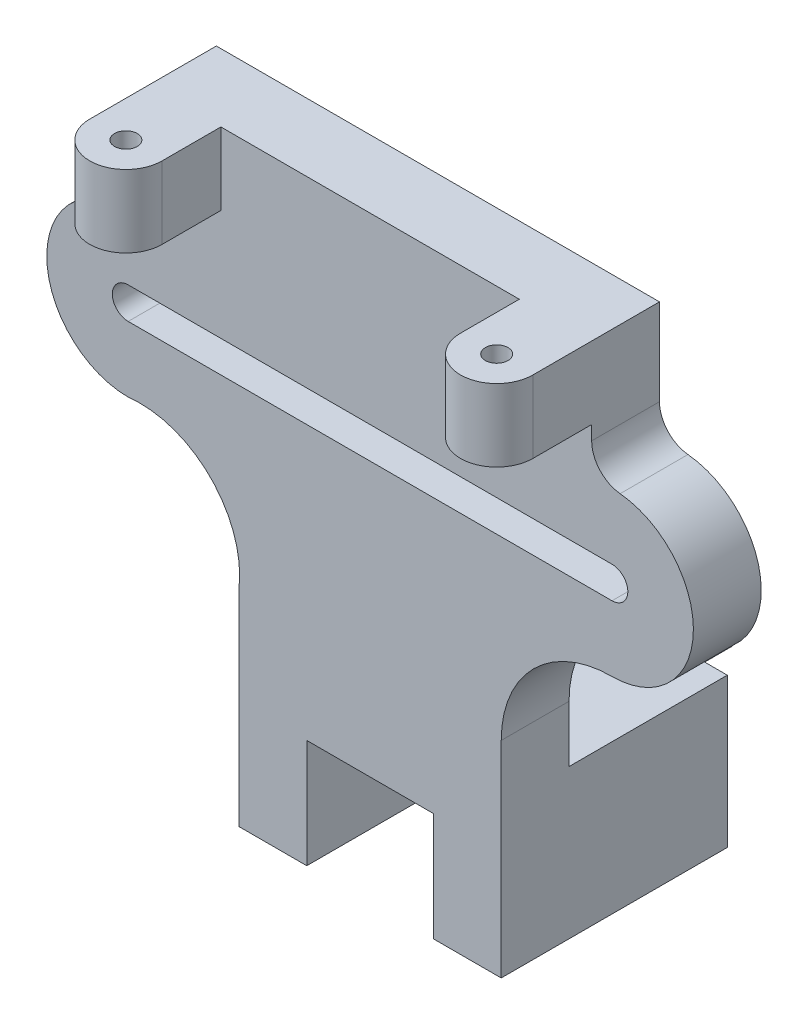
ISO-10303-21;
HEADER;
FILE_DESCRIPTION(('STEP AP214'),'2;1');
FILE_NAME('part.step','',(''),(''),'','','');
FILE_SCHEMA(('AUTOMOTIVE_DESIGN { 1 0 10303 214 1 1 1 1 }'));
ENDSEC;
DATA;
#1=APPLICATION_CONTEXT('core data for automotive mechanical design processes');
#2=APPLICATION_PROTOCOL_DEFINITION('international standard','automotive_design',2000,#1);
#3=PRODUCT_CONTEXT('',#1,'mechanical');
#4=PRODUCT('Part','Part','',(#3));
#5=PRODUCT_RELATED_PRODUCT_CATEGORY('part','',(#4));
#6=PRODUCT_DEFINITION_FORMATION('','',#4);
#7=PRODUCT_DEFINITION_CONTEXT('part definition',#1,'design');
#8=PRODUCT_DEFINITION('design','',#6,#7);
#9=PRODUCT_DEFINITION_SHAPE('','',#8);
#10=(LENGTH_UNIT() NAMED_UNIT(*) SI_UNIT(.MILLI.,.METRE.));
#11=(NAMED_UNIT(*) PLANE_ANGLE_UNIT() SI_UNIT($,.RADIAN.));
#12=(NAMED_UNIT(*) SI_UNIT($,.STERADIAN.) SOLID_ANGLE_UNIT());
#13=UNCERTAINTY_MEASURE_WITH_UNIT(LENGTH_MEASURE(1.E-05),#10,'distance_accuracy_value','');
#14=(GEOMETRIC_REPRESENTATION_CONTEXT(3) GLOBAL_UNCERTAINTY_ASSIGNED_CONTEXT((#13)) GLOBAL_UNIT_ASSIGNED_CONTEXT((#10,
#11,#12)) REPRESENTATION_CONTEXT('',''));
#15=CARTESIAN_POINT('',(0.,0.,0.));
#16=DIRECTION('',(0.,0.,1.));
#17=DIRECTION('',(1.,0.,0.));
#18=AXIS2_PLACEMENT_3D('',#15,#16,#17);
#19=CARTESIAN_POINT('',(0.,0.,0.));
#20=DIRECTION('',(0.,0.,1.));
#21=DIRECTION('',(1.,0.,0.));
#22=AXIS2_PLACEMENT_3D('',#19,#20,#21);
#23=PLANE('',#22);
#24=CARTESIAN_POINT('',(-4.5,-44.,0.));
#25=DIRECTION('',(0.,0.,1.));
#26=DIRECTION('',(1.,0.,0.));
#27=AXIS2_PLACEMENT_3D('',#24,#25,#26);
#28=CIRCLE('',#27,3.5);
#29=CARTESIAN_POINT('',(-4.5,-40.5,0.));
#30=VERTEX_POINT('',#29);
#31=CARTESIAN_POINT('',(-4.5,-47.5,0.));
#32=VERTEX_POINT('',#31);
#33=EDGE_CURVE('E390',#30,#32,#28,.T.);
#34=ORIENTED_EDGE('',*,*,#33,.T.);
#35=DIRECTION('',(1.,0.,0.));
#36=VECTOR('',#35,1.);
#37=CARTESIAN_POINT('',(0.,-47.5,0.));
#38=LINE('',#37,#36);
#39=CARTESIAN_POINT('',(102.5,-47.5,0.));
#40=VERTEX_POINT('',#39);
#41=EDGE_CURVE('E380',#32,#40,#38,.T.);
#42=ORIENTED_EDGE('',*,*,#41,.T.);
#43=CARTESIAN_POINT('',(102.5,-44.,0.));
#44=DIRECTION('',(0.,0.,1.));
#45=DIRECTION('',(1.,0.,0.));
#46=AXIS2_PLACEMENT_3D('',#43,#44,#45);
#47=CIRCLE('',#46,3.50000000000001);
#48=CARTESIAN_POINT('',(102.5,-40.5,0.));
#49=VERTEX_POINT('',#48);
#50=EDGE_CURVE('E379',#40,#49,#47,.T.);
#51=ORIENTED_EDGE('',*,*,#50,.T.);
#52=DIRECTION('',(1.,0.,0.));
#53=VECTOR('',#52,1.);
#54=CARTESIAN_POINT('',(0.,-40.5,0.));
#55=LINE('',#54,#53);
#56=EDGE_CURVE('E383',#30,#49,#55,.T.);
#57=ORIENTED_EDGE('',*,*,#56,.F.);
#58=EDGE_LOOP('',(#34,#42,#51,#57));
#59=FACE_BOUND('',#58,.T.);
#60=DIRECTION('',(0.,1.,0.));
#61=VECTOR('',#60,1.);
#62=CARTESIAN_POINT('',(78.0000000000001,0.,0.));
#63=LINE('',#62,#61);
#64=CARTESIAN_POINT('',(78.,-99.,0.));
#65=VERTEX_POINT('',#64);
#66=CARTESIAN_POINT('',(78.,-86.5,0.));
#67=VERTEX_POINT('',#66);
#68=EDGE_CURVE('E455',#65,#67,#63,.T.);
#69=ORIENTED_EDGE('',*,*,#68,.F.);
#70=DIRECTION('',(-1.,0.,0.));
#71=VECTOR('',#70,1.);
#72=CARTESIAN_POINT('',(0.,-99.,0.));
#73=LINE('',#72,#71);
#74=CARTESIAN_POINT('',(20.,-99.,0.));
#75=VERTEX_POINT('',#74);
#76=EDGE_CURVE('E47',#65,#75,#73,.T.);
#77=ORIENTED_EDGE('',*,*,#76,.T.);
#78=DIRECTION('',(0.,1.,0.));
#79=VECTOR('',#78,1.);
#80=CARTESIAN_POINT('',(20.,0.,0.));
#81=LINE('',#80,#79);
#82=CARTESIAN_POINT('',(20.,-86.5,0.));
#83=VERTEX_POINT('',#82);
#84=EDGE_CURVE('E454',#75,#83,#81,.T.);
#85=ORIENTED_EDGE('',*,*,#84,.T.);
#86=CARTESIAN_POINT('',(-1.83930843846879,-83.8458321587689,0.));
#87=DIRECTION('',(0.,0.,1.));
#88=DIRECTION('',(1.,0.,0.));
#89=AXIS2_PLACEMENT_3D('',#86,#87,#88);
#90=CIRCLE('',#89,22.);
#91=CARTESIAN_POINT('',(-2.16790270932848,-61.8482862546196,0.));
#92=VERTEX_POINT('',#91);
#93=EDGE_CURVE('E450',#92,#83,#90,.F.);
#94=ORIENTED_EDGE('',*,*,#93,.F.);
#95=CARTESIAN_POINT('',(-1.9077841989313,-83.8467484363392,0.));
#96=DIRECTION('',(0.,0.,1.));
#97=DIRECTION('',(1.,0.,0.));
#98=AXIS2_PLACEMENT_3D('',#95,#96,#97);
#99=CIRCLE('',#98,22.);
#100=CARTESIAN_POINT('',(-4.49999999999998,-62.,0.));
#101=VERTEX_POINT('',#100);
#102=EDGE_CURVE('E405',#101,#92,#99,.F.);
#103=ORIENTED_EDGE('',*,*,#102,.F.);
#104=CARTESIAN_POINT('',(-4.5,-44.,0.));
#105=DIRECTION('',(0.,0.,1.));
#106=DIRECTION('',(1.,0.,0.));
#107=AXIS2_PLACEMENT_3D('',#104,#105,#106);
#108=CIRCLE('',#107,18.);
#109=CARTESIAN_POINT('',(-6.3,-26.0902261320808,0.));
#110=VERTEX_POINT('',#109);
#111=EDGE_CURVE('E415',#110,#101,#108,.T.);
#112=ORIENTED_EDGE('',*,*,#111,.F.);
#113=CARTESIAN_POINT('',(-7.,-19.1253140723345,0.));
#114=DIRECTION('',(0.,0.,1.));
#115=DIRECTION('',(1.,0.,0.));
#116=AXIS2_PLACEMENT_3D('',#113,#114,#115);
#117=CIRCLE('',#116,7.);
#118=CARTESIAN_POINT('',(0.,-19.1253140723345,0.));
#119=VERTEX_POINT('',#118);
#120=EDGE_CURVE('E472',#110,#119,#117,.T.);
#121=ORIENTED_EDGE('',*,*,#120,.T.);
#122=DIRECTION('',(0.,-1.,0.));
#123=VECTOR('',#122,1.);
#124=CARTESIAN_POINT('',(0.,0.,0.));
#125=LINE('',#124,#123);
#126=CARTESIAN_POINT('',(0.,0.,0.));
#127=VERTEX_POINT('',#126);
#128=EDGE_CURVE('E468',#127,#119,#125,.T.);
#129=ORIENTED_EDGE('',*,*,#128,.F.);
#130=DIRECTION('',(1.,0.,0.));
#131=VECTOR('',#130,1.);
#132=CARTESIAN_POINT('',(0.,0.,0.));
#133=LINE('',#132,#131);
#134=CARTESIAN_POINT('',(98.,0.,0.));
#135=VERTEX_POINT('',#134);
#136=EDGE_CURVE('E469',#127,#135,#133,.T.);
#137=ORIENTED_EDGE('',*,*,#136,.T.);
#138=DIRECTION('',(0.,-1.,0.));
#139=VECTOR('',#138,1.);
#140=CARTESIAN_POINT('',(98.,0.,0.));
#141=LINE('',#140,#139);
#142=CARTESIAN_POINT('',(98.,-19.1253140723345,0.));
#143=VERTEX_POINT('',#142);
#144=EDGE_CURVE('E465',#135,#143,#141,.T.);
#145=ORIENTED_EDGE('',*,*,#144,.T.);
#146=CARTESIAN_POINT('',(105.,-19.1253140723345,0.));
#147=DIRECTION('',(0.,0.,1.));
#148=DIRECTION('',(1.,0.,0.));
#149=AXIS2_PLACEMENT_3D('',#146,#147,#148);
#150=CIRCLE('',#149,7.);
#151=CARTESIAN_POINT('',(104.3,-26.0902261320808,0.));
#152=VERTEX_POINT('',#151);
#153=EDGE_CURVE('E458',#152,#143,#150,.F.);
#154=ORIENTED_EDGE('',*,*,#153,.F.);
#155=CARTESIAN_POINT('',(102.5,-44.,0.));
#156=DIRECTION('',(0.,0.,1.));
#157=DIRECTION('',(1.,0.,0.));
#158=AXIS2_PLACEMENT_3D('',#155,#156,#157);
#159=CIRCLE('',#158,18.);
#160=CARTESIAN_POINT('',(102.5,-62.,0.));
#161=VERTEX_POINT('',#160);
#162=EDGE_CURVE('E456',#161,#152,#159,.T.);
#163=ORIENTED_EDGE('',*,*,#162,.F.);
#164=CARTESIAN_POINT('',(102.5,-86.5,0.));
#165=DIRECTION('',(0.,0.,1.));
#166=DIRECTION('',(1.,0.,0.));
#167=AXIS2_PLACEMENT_3D('',#164,#165,#166);
#168=CIRCLE('',#167,24.5);
#169=EDGE_CURVE('E452',#161,#67,#168,.T.);
#170=ORIENTED_EDGE('',*,*,#169,.T.);
#171=EDGE_LOOP('',(#69,#77,#85,#94,#103,#112,#121,#129,#137,#145,#154,#163,#170));
#172=FACE_BOUND('',#171,.T.);
#173=ADVANCED_FACE('F41',(#59,#172),#23,.F.);
#174=CARTESIAN_POINT('',(35.,0.,0.));
#175=DIRECTION('',(-1.,0.,0.));
#176=DIRECTION('',(0.,-1.,0.));
#177=AXIS2_PLACEMENT_3D('',#174,#175,#176);
#178=PLANE('',#177);
#179=DIRECTION('',(0.,1.,0.));
#180=VECTOR('',#179,1.);
#181=CARTESIAN_POINT('',(35.,-108.,-50.));
#182=LINE('',#181,#180);
#183=CARTESIAN_POINT('',(35.,-108.,-50.));
#184=VERTEX_POINT('',#183);
#185=CARTESIAN_POINT('',(35.,-99.,-50.));
#186=VERTEX_POINT('',#185);
#187=EDGE_CURVE('E333',#184,#186,#182,.T.);
#188=ORIENTED_EDGE('',*,*,#187,.F.);
#189=DIRECTION('',(0.,0.,1.));
#190=VECTOR('',#189,1.);
#191=CARTESIAN_POINT('',(35.,-108.,15.));
#192=LINE('',#191,#190);
#193=CARTESIAN_POINT('',(35.,-108.,15.));
#194=VERTEX_POINT('',#193);
#195=EDGE_CURVE('E371',#184,#194,#192,.T.);
#196=ORIENTED_EDGE('',*,*,#195,.T.);
#197=DIRECTION('',(0.,1.,0.));
#198=VECTOR('',#197,1.);
#199=CARTESIAN_POINT('',(35.,-132.,15.));
#200=LINE('',#199,#198);
#201=CARTESIAN_POINT('',(35.,-132.,15.));
#202=VERTEX_POINT('',#201);
#203=EDGE_CURVE('E353',#202,#194,#200,.T.);
#204=ORIENTED_EDGE('',*,*,#203,.F.);
#205=DIRECTION('',(0.,0.,1.));
#206=VECTOR('',#205,1.);
#207=CARTESIAN_POINT('',(35.,-132.,-51.));
#208=LINE('',#207,#206);
#209=CARTESIAN_POINT('',(35.,-132.,-51.));
#210=VERTEX_POINT('',#209);
#211=EDGE_CURVE('E354',#210,#202,#208,.T.);
#212=ORIENTED_EDGE('',*,*,#211,.F.);
#213=DIRECTION('',(0.,-1.,0.));
#214=VECTOR('',#213,1.);
#215=CARTESIAN_POINT('',(35.,-99.,-51.));
#216=LINE('',#215,#214);
#217=CARTESIAN_POINT('',(35.,-99.,-51.));
#218=VERTEX_POINT('',#217);
#219=EDGE_CURVE('E363',#218,#210,#216,.T.);
#220=ORIENTED_EDGE('',*,*,#219,.F.);
#221=DIRECTION('',(0.,0.,-1.));
#222=VECTOR('',#221,1.);
#223=CARTESIAN_POINT('',(35.,-99.,15.));
#224=LINE('',#223,#222);
#225=EDGE_CURVE('E358',#186,#218,#224,.T.);
#226=ORIENTED_EDGE('',*,*,#225,.F.);
#227=EDGE_LOOP('',(#188,#196,#204,#212,#220,#226));
#228=FACE_BOUND('',#227,.T.);
#229=ADVANCED_FACE('F585',(#228),#178,.F.);
#230=CARTESIAN_POINT('',(0.,-108.,15.));
#231=DIRECTION('',(0.,1.,0.));
#232=DIRECTION('',(0.,0.,1.));
#233=AXIS2_PLACEMENT_3D('',#230,#231,#232);
#234=PLANE('',#233);
#235=DIRECTION('',(0.,0.,1.));
#236=VECTOR('',#235,1.);
#237=CARTESIAN_POINT('',(64.,-108.,-50.));
#238=LINE('',#237,#236);
#239=CARTESIAN_POINT('',(64.,-108.,-50.));
#240=VERTEX_POINT('',#239);
#241=CARTESIAN_POINT('',(64.,-108.,-35.));
#242=VERTEX_POINT('',#241);
#243=EDGE_CURVE('E342',#240,#242,#238,.T.);
#244=ORIENTED_EDGE('',*,*,#243,.T.);
#245=DIRECTION('',(-1.,0.,0.));
#246=VECTOR('',#245,1.);
#247=CARTESIAN_POINT('',(0.,-108.,-35.));
#248=LINE('',#247,#246);
#249=CARTESIAN_POINT('',(63.,-108.,-35.));
#250=VERTEX_POINT('',#249);
#251=EDGE_CURVE('E330',#242,#250,#248,.T.);
#252=ORIENTED_EDGE('',*,*,#251,.T.);
#253=DIRECTION('',(0.,0.,1.));
#254=VECTOR('',#253,1.);
#255=CARTESIAN_POINT('',(63.,-108.,15.));
#256=LINE('',#255,#254);
#257=CARTESIAN_POINT('',(63.,-108.,15.));
#258=VERTEX_POINT('',#257);
#259=EDGE_CURVE('E335',#250,#258,#256,.T.);
#260=ORIENTED_EDGE('',*,*,#259,.T.);
#261=DIRECTION('',(1.,0.,0.));
#262=VECTOR('',#261,1.);
#263=CARTESIAN_POINT('',(0.,-108.,15.));
#264=LINE('',#263,#262);
#265=EDGE_CURVE('E419',#194,#258,#264,.T.);
#266=ORIENTED_EDGE('',*,*,#265,.F.);
#267=ORIENTED_EDGE('',*,*,#195,.F.);
#268=DIRECTION('',(-1.,0.,0.));
#269=VECTOR('',#268,1.);
#270=CARTESIAN_POINT('',(64.,-108.,-50.));
#271=LINE('',#270,#269);
#272=EDGE_CURVE('E341',#240,#184,#271,.T.);
#273=ORIENTED_EDGE('',*,*,#272,.F.);
#274=EDGE_LOOP('',(#244,#252,#260,#266,#267,#273));
#275=FACE_BOUND('',#274,.T.);
#276=ADVANCED_FACE('F590',(#275),#234,.F.);
#277=CARTESIAN_POINT('',(-1.9077841989313,-83.8467484363392,15.));
#278=DIRECTION('',(0.,0.,-1.));
#279=DIRECTION('',(-1.,0.,0.));
#280=AXIS2_PLACEMENT_3D('',#277,#278,#279);
#281=CYLINDRICAL_SURFACE('',#280,22.);
#282=ORIENTED_EDGE('',*,*,#102,.T.);
#283=DIRECTION('',(0.,0.,-1.));
#284=VECTOR('',#283,1.);
#285=CARTESIAN_POINT('',(-2.16790270932848,-61.8482862546196,15.));
#286=LINE('',#285,#284);
#287=CARTESIAN_POINT('',(-2.16790270932848,-61.8482862546196,15.));
#288=VERTEX_POINT('',#287);
#289=EDGE_CURVE('E505',#288,#92,#286,.T.);
#290=ORIENTED_EDGE('',*,*,#289,.F.);
#291=CARTESIAN_POINT('',(-1.9077841989313,-83.8467484363392,15.));
#292=DIRECTION('',(0.,0.,1.));
#293=DIRECTION('',(1.,0.,0.));
#294=AXIS2_PLACEMENT_3D('',#291,#292,#293);
#295=CIRCLE('',#294,22.);
#296=CARTESIAN_POINT('',(-4.49999999999998,-62.,15.));
#297=VERTEX_POINT('',#296);
#298=EDGE_CURVE('E406',#297,#288,#295,.F.);
#299=ORIENTED_EDGE('',*,*,#298,.F.);
#300=DIRECTION('',(0.,0.,-1.));
#301=VECTOR('',#300,1.);
#302=CARTESIAN_POINT('',(-4.49999999999998,-62.,15.));
#303=LINE('',#302,#301);
#304=EDGE_CURVE('E443',#297,#101,#303,.T.);
#305=ORIENTED_EDGE('',*,*,#304,.T.);
#306=EDGE_LOOP('',(#282,#290,#299,#305));
#307=FACE_BOUND('',#306,.T.);
#308=ADVANCED_FACE('F43',(#307),#281,.F.);
#309=CARTESIAN_POINT('',(-1.83930843846879,-83.8458321587689,15.));
#310=DIRECTION('',(0.,0.,-1.));
#311=DIRECTION('',(-1.,0.,0.));
#312=AXIS2_PLACEMENT_3D('',#309,#310,#311);
#313=CYLINDRICAL_SURFACE('',#312,22.);
#314=ORIENTED_EDGE('',*,*,#93,.T.);
#315=DIRECTION('',(0.,0.,-1.));
#316=VECTOR('',#315,1.);
#317=CARTESIAN_POINT('',(20.,-86.5,15.));
#318=LINE('',#317,#316);
#319=CARTESIAN_POINT('',(20.,-86.5,15.));
#320=VERTEX_POINT('',#319);
#321=EDGE_CURVE('E498',#320,#83,#318,.T.);
#322=ORIENTED_EDGE('',*,*,#321,.F.);
#323=CARTESIAN_POINT('',(-1.83930843846879,-83.8458321587689,15.));
#324=DIRECTION('',(0.,0.,1.));
#325=DIRECTION('',(1.,0.,0.));
#326=AXIS2_PLACEMENT_3D('',#323,#324,#325);
#327=CIRCLE('',#326,22.);
#328=EDGE_CURVE('E411',#288,#320,#327,.F.);
#329=ORIENTED_EDGE('',*,*,#328,.F.);
#330=ORIENTED_EDGE('',*,*,#289,.T.);
#331=EDGE_LOOP('',(#314,#322,#329,#330));
#332=FACE_BOUND('',#331,.T.);
#333=ADVANCED_FACE('F531',(#332),#313,.F.);
#334=CARTESIAN_POINT('',(20.,0.,15.));
#335=DIRECTION('',(-1.,0.,0.));
#336=DIRECTION('',(0.,-1.,0.));
#337=AXIS2_PLACEMENT_3D('',#334,#335,#336);
#338=PLANE('',#337);
#339=ORIENTED_EDGE('',*,*,#84,.F.);
#340=DIRECTION('',(0.,0.,-1.));
#341=VECTOR('',#340,1.);
#342=CARTESIAN_POINT('',(20.,-99.,15.));
#343=LINE('',#342,#341);
#344=CARTESIAN_POINT('',(20.,-99.,-51.));
#345=VERTEX_POINT('',#344);
#346=EDGE_CURVE('E352',#75,#345,#343,.T.);
#347=ORIENTED_EDGE('',*,*,#346,.T.);
#348=DIRECTION('',(0.,-1.,0.));
#349=VECTOR('',#348,1.);
#350=CARTESIAN_POINT('',(20.,-99.,-51.));
#351=LINE('',#350,#349);
#352=CARTESIAN_POINT('',(20.,-132.,-51.));
#353=VERTEX_POINT('',#352);
#354=EDGE_CURVE('E359',#345,#353,#351,.T.);
#355=ORIENTED_EDGE('',*,*,#354,.T.);
#356=DIRECTION('',(0.,0.,-1.));
#357=VECTOR('',#356,1.);
#358=CARTESIAN_POINT('',(20.,-132.,15.));
#359=LINE('',#358,#357);
#360=CARTESIAN_POINT('',(20.,-132.,15.));
#361=VERTEX_POINT('',#360);
#362=EDGE_CURVE('E499',#361,#353,#359,.T.);
#363=ORIENTED_EDGE('',*,*,#362,.F.);
#364=DIRECTION('',(0.,1.,0.));
#365=VECTOR('',#364,1.);
#366=CARTESIAN_POINT('',(20.,0.,15.));
#367=LINE('',#366,#365);
#368=EDGE_CURVE('E418',#361,#320,#367,.T.);
#369=ORIENTED_EDGE('',*,*,#368,.T.);
#370=ORIENTED_EDGE('',*,*,#321,.T.);
#371=EDGE_LOOP('',(#339,#347,#355,#363,#369,#370));
#372=FACE_BOUND('',#371,.T.);
#373=ADVANCED_FACE('F515',(#372),#338,.T.);
#374=CARTESIAN_POINT('',(0.,-132.,15.));
#375=DIRECTION('',(0.,1.,0.));
#376=DIRECTION('',(0.,0.,1.));
#377=AXIS2_PLACEMENT_3D('',#374,#375,#376);
#378=PLANE('',#377);
#379=ORIENTED_EDGE('',*,*,#362,.T.);
#380=DIRECTION('',(-1.,0.,0.));
#381=VECTOR('',#380,1.);
#382=CARTESIAN_POINT('',(35.,-132.,-51.));
#383=LINE('',#382,#381);
#384=EDGE_CURVE('E366',#210,#353,#383,.T.);
#385=ORIENTED_EDGE('',*,*,#384,.F.);
#386=ORIENTED_EDGE('',*,*,#211,.T.);
#387=DIRECTION('',(1.,0.,0.));
#388=VECTOR('',#387,1.);
#389=CARTESIAN_POINT('',(0.,-132.,15.));
#390=LINE('',#389,#388);
#391=EDGE_CURVE('E416',#361,#202,#390,.T.);
#392=ORIENTED_EDGE('',*,*,#391,.F.);
#393=EDGE_LOOP('',(#379,#385,#386,#392));
#394=FACE_BOUND('',#393,.T.);
#395=ADVANCED_FACE('F522',(#394),#378,.F.);
#396=CARTESIAN_POINT('',(0.,-132.,15.));
#397=DIRECTION('',(0.,1.,0.));
#398=DIRECTION('',(0.,0.,1.));
#399=AXIS2_PLACEMENT_3D('',#396,#397,#398);
#400=PLANE('',#399);
#401=DIRECTION('',(1.,0.,0.));
#402=VECTOR('',#401,1.);
#403=CARTESIAN_POINT('',(63.,-132.,-35.));
#404=LINE('',#403,#402);
#405=CARTESIAN_POINT('',(63.,-132.,-35.));
#406=VERTEX_POINT('',#405);
#407=CARTESIAN_POINT('',(78.,-132.,-35.));
#408=VERTEX_POINT('',#407);
#409=EDGE_CURVE('E319',#406,#408,#404,.T.);
#410=ORIENTED_EDGE('',*,*,#409,.T.);
#411=DIRECTION('',(0.,0.,-1.));
#412=VECTOR('',#411,1.);
#413=CARTESIAN_POINT('',(78.,-132.,15.));
#414=LINE('',#413,#412);
#415=CARTESIAN_POINT('',(78.,-132.,15.));
#416=VERTEX_POINT('',#415);
#417=EDGE_CURVE('E497',#416,#408,#414,.T.);
#418=ORIENTED_EDGE('',*,*,#417,.F.);
#419=DIRECTION('',(1.,0.,0.));
#420=VECTOR('',#419,1.);
#421=CARTESIAN_POINT('',(0.,-132.,15.));
#422=LINE('',#421,#420);
#423=CARTESIAN_POINT('',(63.,-132.,15.));
#424=VERTEX_POINT('',#423);
#425=EDGE_CURVE('E421',#424,#416,#422,.T.);
#426=ORIENTED_EDGE('',*,*,#425,.F.);
#427=DIRECTION('',(0.,0.,-1.));
#428=VECTOR('',#427,1.);
#429=CARTESIAN_POINT('',(63.,-132.,-35.));
#430=LINE('',#429,#428);
#431=EDGE_CURVE('E309',#424,#406,#430,.T.);
#432=ORIENTED_EDGE('',*,*,#431,.T.);
#433=EDGE_LOOP('',(#410,#418,#426,#432));
#434=FACE_BOUND('',#433,.T.);
#435=ADVANCED_FACE('F592',(#434),#400,.F.);
#436=CARTESIAN_POINT('',(78.0000000000001,0.,15.));
#437=DIRECTION('',(-1.,0.,0.));
#438=DIRECTION('',(0.,-1.,0.));
#439=AXIS2_PLACEMENT_3D('',#436,#437,#438);
#440=PLANE('',#439);
#441=DIRECTION('',(0.,0.,-1.));
#442=VECTOR('',#441,1.);
#443=CARTESIAN_POINT('',(78.,-86.5,15.));
#444=LINE('',#443,#442);
#445=CARTESIAN_POINT('',(78.,-86.5,15.));
#446=VERTEX_POINT('',#445);
#447=EDGE_CURVE('E492',#446,#67,#444,.T.);
#448=ORIENTED_EDGE('',*,*,#447,.F.);
#449=DIRECTION('',(0.,1.,0.));
#450=VECTOR('',#449,1.);
#451=CARTESIAN_POINT('',(78.0000000000001,0.,15.));
#452=LINE('',#451,#450);
#453=EDGE_CURVE('E422',#416,#446,#452,.T.);
#454=ORIENTED_EDGE('',*,*,#453,.F.);
#455=ORIENTED_EDGE('',*,*,#417,.T.);
#456=DIRECTION('',(0.,1.,0.));
#457=VECTOR('',#456,1.);
#458=CARTESIAN_POINT('',(78.,-99.,-35.));
#459=LINE('',#458,#457);
#460=CARTESIAN_POINT('',(78.,-99.,-35.));
#461=VERTEX_POINT('',#460);
#462=EDGE_CURVE('E302',#408,#461,#459,.T.);
#463=ORIENTED_EDGE('',*,*,#462,.T.);
#464=DIRECTION('',(0.,0.,1.));
#465=VECTOR('',#464,1.);
#466=CARTESIAN_POINT('',(78.,-99.,15.));
#467=LINE('',#466,#465);
#468=EDGE_CURVE('E314',#461,#65,#467,.T.);
#469=ORIENTED_EDGE('',*,*,#468,.T.);
#470=ORIENTED_EDGE('',*,*,#68,.T.);
#471=EDGE_LOOP('',(#448,#454,#455,#463,#469,#470));
#472=FACE_BOUND('',#471,.T.);
#473=ADVANCED_FACE('F572',(#472),#440,.F.);
#474=CARTESIAN_POINT('',(102.5,-86.5,15.));
#475=DIRECTION('',(0.,0.,-1.));
#476=DIRECTION('',(-1.,0.,0.));
#477=AXIS2_PLACEMENT_3D('',#474,#475,#476);
#478=CYLINDRICAL_SURFACE('',#477,24.5);
#479=ORIENTED_EDGE('',*,*,#169,.F.);
#480=DIRECTION('',(0.,0.,-1.));
#481=VECTOR('',#480,1.);
#482=CARTESIAN_POINT('',(102.5,-62.,15.));
#483=LINE('',#482,#481);
#484=CARTESIAN_POINT('',(102.5,-62.,15.));
#485=VERTEX_POINT('',#484);
#486=EDGE_CURVE('E491',#485,#161,#483,.T.);
#487=ORIENTED_EDGE('',*,*,#486,.F.);
#488=CARTESIAN_POINT('',(102.5,-86.5,15.));
#489=DIRECTION('',(0.,0.,1.));
#490=DIRECTION('',(1.,0.,0.));
#491=AXIS2_PLACEMENT_3D('',#488,#489,#490);
#492=CIRCLE('',#491,24.5);
#493=EDGE_CURVE('E430',#485,#446,#492,.T.);
#494=ORIENTED_EDGE('',*,*,#493,.T.);
#495=ORIENTED_EDGE('',*,*,#447,.T.);
#496=EDGE_LOOP('',(#479,#487,#494,#495));
#497=FACE_BOUND('',#496,.T.);
#498=ADVANCED_FACE('F570',(#497),#478,.F.);
#499=CARTESIAN_POINT('',(102.5,-44.,15.));
#500=DIRECTION('',(0.,0.,-1.));
#501=DIRECTION('',(-1.,0.,0.));
#502=AXIS2_PLACEMENT_3D('',#499,#500,#501);
#503=CYLINDRICAL_SURFACE('',#502,18.);
#504=ORIENTED_EDGE('',*,*,#162,.T.);
#505=DIRECTION('',(0.,0.,-1.));
#506=VECTOR('',#505,1.);
#507=CARTESIAN_POINT('',(104.3,-26.0902261320808,15.));
#508=LINE('',#507,#506);
#509=CARTESIAN_POINT('',(104.3,-26.0902261320808,15.));
#510=VERTEX_POINT('',#509);
#511=EDGE_CURVE('E488',#510,#152,#508,.T.);
#512=ORIENTED_EDGE('',*,*,#511,.F.);
#513=CARTESIAN_POINT('',(102.5,-44.,15.));
#514=DIRECTION('',(0.,0.,1.));
#515=DIRECTION('',(1.,0.,0.));
#516=AXIS2_PLACEMENT_3D('',#513,#514,#515);
#517=CIRCLE('',#516,18.);
#518=EDGE_CURVE('E429',#485,#510,#517,.T.);
#519=ORIENTED_EDGE('',*,*,#518,.F.);
#520=ORIENTED_EDGE('',*,*,#486,.T.);
#521=EDGE_LOOP('',(#504,#512,#519,#520));
#522=FACE_BOUND('',#521,.T.);
#523=ADVANCED_FACE('F563',(#522),#503,.T.);
#524=CARTESIAN_POINT('',(105.,-19.1253140723345,15.));
#525=DIRECTION('',(0.,0.,-1.));
#526=DIRECTION('',(-1.,0.,0.));
#527=AXIS2_PLACEMENT_3D('',#524,#525,#526);
#528=CYLINDRICAL_SURFACE('',#527,7.);
#529=ORIENTED_EDGE('',*,*,#153,.T.);
#530=DIRECTION('',(0.,0.,-1.));
#531=VECTOR('',#530,1.);
#532=CARTESIAN_POINT('',(98.,-19.1253140723345,15.));
#533=LINE('',#532,#531);
#534=CARTESIAN_POINT('',(98.,-19.1253140723345,15.));
#535=VERTEX_POINT('',#534);
#536=EDGE_CURVE('E486',#535,#143,#533,.T.);
#537=ORIENTED_EDGE('',*,*,#536,.F.);
#538=CARTESIAN_POINT('',(105.,-19.1253140723345,15.));
#539=DIRECTION('',(0.,0.,1.));
#540=DIRECTION('',(1.,0.,0.));
#541=AXIS2_PLACEMENT_3D('',#538,#539,#540);
#542=CIRCLE('',#541,7.);
#543=EDGE_CURVE('E435',#510,#535,#542,.F.);
#544=ORIENTED_EDGE('',*,*,#543,.F.);
#545=ORIENTED_EDGE('',*,*,#511,.T.);
#546=EDGE_LOOP('',(#529,#537,#544,#545));
#547=FACE_BOUND('',#546,.T.);
#548=ADVANCED_FACE('F556',(#547),#528,.F.);
#549=CARTESIAN_POINT('',(98.,0.,15.));
#550=DIRECTION('',(1.,0.,0.));
#551=DIRECTION('',(0.,0.,-1.));
#552=AXIS2_PLACEMENT_3D('',#549,#550,#551);
#553=PLANE('',#552);
#554=ORIENTED_EDGE('',*,*,#144,.F.);
#555=DIRECTION('',(0.,0.,-1.));
#556=VECTOR('',#555,1.);
#557=CARTESIAN_POINT('',(98.,0.,15.));
#558=LINE('',#557,#556);
#559=CARTESIAN_POINT('',(98.,0.,28.));
#560=VERTEX_POINT('',#559);
#561=EDGE_CURVE('E482',#560,#135,#558,.T.);
#562=ORIENTED_EDGE('',*,*,#561,.F.);
#563=DIRECTION('',(0.,1.,0.));
#564=VECTOR('',#563,1.);
#565=CARTESIAN_POINT('',(98.,-16.,28.));
#566=LINE('',#565,#564);
#567=CARTESIAN_POINT('',(98.,-16.,28.));
#568=VERTEX_POINT('',#567);
#569=EDGE_CURVE('E257',#568,#560,#566,.T.);
#570=ORIENTED_EDGE('',*,*,#569,.F.);
#571=DIRECTION('',(0.,0.,1.));
#572=VECTOR('',#571,1.);
#573=CARTESIAN_POINT('',(98.,-16.,1.0461716962814E-13));
#574=LINE('',#573,#572);
#575=CARTESIAN_POINT('',(98.,-16.,15.));
#576=VERTEX_POINT('',#575);
#577=EDGE_CURVE('E267',#576,#568,#574,.T.);
#578=ORIENTED_EDGE('',*,*,#577,.F.);
#579=DIRECTION('',(0.,-1.,0.));
#580=VECTOR('',#579,1.);
#581=CARTESIAN_POINT('',(98.,0.,15.));
#582=LINE('',#581,#580);
#583=EDGE_CURVE('E434',#576,#535,#582,.T.);
#584=ORIENTED_EDGE('',*,*,#583,.T.);
#585=ORIENTED_EDGE('',*,*,#536,.T.);
#586=EDGE_LOOP('',(#554,#562,#570,#578,#584,#585));
#587=FACE_BOUND('',#586,.T.);
#588=ADVANCED_FACE('F554',(#587),#553,.T.);
#589=CARTESIAN_POINT('',(0.,0.,15.));
#590=DIRECTION('',(0.,1.,0.));
#591=DIRECTION('',(0.,0.,1.));
#592=AXIS2_PLACEMENT_3D('',#589,#590,#591);
#593=PLANE('',#592);
#594=CARTESIAN_POINT('',(90.,0.,28.));
#595=DIRECTION('',(0.,-1.,0.));
#596=DIRECTION('',(0.,0.,-1.));
#597=AXIS2_PLACEMENT_3D('',#594,#595,#596);
#598=CIRCLE('',#597,2.49999999999999);
#599=CARTESIAN_POINT('',(90.,0.,25.5));
#600=VERTEX_POINT('',#599);
#601=EDGE_CURVE('E285',#600,#600,#598,.T.);
#602=ORIENTED_EDGE('',*,*,#601,.T.);
#603=EDGE_LOOP('',(#602));
#604=FACE_BOUND('',#603,.T.);
#605=CARTESIAN_POINT('',(8.,0.,28.));
#606=DIRECTION('',(0.,-1.,0.));
#607=DIRECTION('',(0.,0.,-1.));
#608=AXIS2_PLACEMENT_3D('',#605,#606,#607);
#609=CIRCLE('',#608,2.5);
#610=CARTESIAN_POINT('',(8.,0.,25.5));
#611=VERTEX_POINT('',#610);
#612=EDGE_CURVE('E962',#611,#611,#609,.T.);
#613=ORIENTED_EDGE('',*,*,#612,.T.);
#614=EDGE_LOOP('',(#613));
#615=FACE_BOUND('',#614,.T.);
#616=ORIENTED_EDGE('',*,*,#136,.F.);
#617=DIRECTION('',(0.,0.,-1.));
#618=VECTOR('',#617,1.);
#619=CARTESIAN_POINT('',(0.,0.,15.));
#620=LINE('',#619,#618);
#621=CARTESIAN_POINT('',(0.,0.,28.));
#622=VERTEX_POINT('',#621);
#623=EDGE_CURVE('E485',#622,#127,#620,.T.);
#624=ORIENTED_EDGE('',*,*,#623,.F.);
#625=CARTESIAN_POINT('',(8.,0.,28.));
#626=DIRECTION('',(0.,1.,0.));
#627=DIRECTION('',(0.,0.,1.));
#628=AXIS2_PLACEMENT_3D('',#625,#626,#627);
#629=CIRCLE('',#628,8.);
#630=CARTESIAN_POINT('',(16.,0.,28.));
#631=VERTEX_POINT('',#630);
#632=EDGE_CURVE('E289',#622,#631,#629,.T.);
#633=ORIENTED_EDGE('',*,*,#632,.T.);
#634=DIRECTION('',(0.,0.,1.));
#635=VECTOR('',#634,1.);
#636=CARTESIAN_POINT('',(16.,0.,0.));
#637=LINE('',#636,#635);
#638=CARTESIAN_POINT('',(16.,0.,15.));
#639=VERTEX_POINT('',#638);
#640=EDGE_CURVE('E295',#639,#631,#637,.T.);
#641=ORIENTED_EDGE('',*,*,#640,.F.);
#642=DIRECTION('',(1.,0.,0.));
#643=VECTOR('',#642,1.);
#644=CARTESIAN_POINT('',(0.,0.,15.));
#645=LINE('',#644,#643);
#646=CARTESIAN_POINT('',(82.,0.,15.));
#647=VERTEX_POINT('',#646);
#648=EDGE_CURVE('E64',#639,#647,#645,.T.);
#649=ORIENTED_EDGE('',*,*,#648,.T.);
#650=DIRECTION('',(0.,0.,1.));
#651=VECTOR('',#650,1.);
#652=CARTESIAN_POINT('',(82.,0.,0.));
#653=LINE('',#652,#651);
#654=CARTESIAN_POINT('',(82.,0.,28.));
#655=VERTEX_POINT('',#654);
#656=EDGE_CURVE('E274',#647,#655,#653,.T.);
#657=ORIENTED_EDGE('',*,*,#656,.T.);
#658=CARTESIAN_POINT('',(90.,0.,28.));
#659=DIRECTION('',(0.,1.,0.));
#660=DIRECTION('',(0.,0.,1.));
#661=AXIS2_PLACEMENT_3D('',#658,#659,#660);
#662=CIRCLE('',#661,7.99999999999999);
#663=EDGE_CURVE('E258',#655,#560,#662,.T.);
#664=ORIENTED_EDGE('',*,*,#663,.T.);
#665=ORIENTED_EDGE('',*,*,#561,.T.);
#666=EDGE_LOOP('',(#616,#624,#633,#641,#649,#657,#664,#665));
#667=FACE_BOUND('',#666,.T.);
#668=ADVANCED_FACE('F549',(#604,#615,#667),#593,.T.);
#669=CARTESIAN_POINT('',(0.,0.,15.));
#670=DIRECTION('',(1.,0.,0.));
#671=DIRECTION('',(0.,0.,-1.));
#672=AXIS2_PLACEMENT_3D('',#669,#670,#671);
#673=PLANE('',#672);
#674=ORIENTED_EDGE('',*,*,#128,.T.);
#675=DIRECTION('',(0.,0.,-1.));
#676=VECTOR('',#675,1.);
#677=CARTESIAN_POINT('',(0.,-19.1253140723345,15.));
#678=LINE('',#677,#676);
#679=CARTESIAN_POINT('',(0.,-19.1253140723345,15.));
#680=VERTEX_POINT('',#679);
#681=EDGE_CURVE('E477',#680,#119,#678,.T.);
#682=ORIENTED_EDGE('',*,*,#681,.F.);
#683=DIRECTION('',(0.,-1.,0.));
#684=VECTOR('',#683,1.);
#685=CARTESIAN_POINT('',(0.,0.,15.));
#686=LINE('',#685,#684);
#687=CARTESIAN_POINT('',(0.,-16.,15.));
#688=VERTEX_POINT('',#687);
#689=EDGE_CURVE('E437',#688,#680,#686,.T.);
#690=ORIENTED_EDGE('',*,*,#689,.F.);
#691=DIRECTION('',(0.,0.,1.));
#692=VECTOR('',#691,1.);
#693=CARTESIAN_POINT('',(0.,-16.,0.));
#694=LINE('',#693,#692);
#695=CARTESIAN_POINT('',(0.,-16.,28.));
#696=VERTEX_POINT('',#695);
#697=EDGE_CURVE('E290',#688,#696,#694,.T.);
#698=ORIENTED_EDGE('',*,*,#697,.T.);
#699=DIRECTION('',(0.,1.,0.));
#700=VECTOR('',#699,1.);
#701=CARTESIAN_POINT('',(0.,-16.,28.));
#702=LINE('',#701,#700);
#703=EDGE_CURVE('E300',#696,#622,#702,.T.);
#704=ORIENTED_EDGE('',*,*,#703,.T.);
#705=ORIENTED_EDGE('',*,*,#623,.T.);
#706=EDGE_LOOP('',(#674,#682,#690,#698,#704,#705));
#707=FACE_BOUND('',#706,.T.);
#708=ADVANCED_FACE('F607',(#707),#673,.F.);
#709=CARTESIAN_POINT('',(-7.,-19.1253140723345,15.));
#710=DIRECTION('',(0.,0.,-1.));
#711=DIRECTION('',(-1.,0.,0.));
#712=AXIS2_PLACEMENT_3D('',#709,#710,#711);
#713=CYLINDRICAL_SURFACE('',#712,7.);
#714=ORIENTED_EDGE('',*,*,#120,.F.);
#715=DIRECTION('',(0.,0.,-1.));
#716=VECTOR('',#715,1.);
#717=CARTESIAN_POINT('',(-6.3,-26.0902261320808,15.));
#718=LINE('',#717,#716);
#719=CARTESIAN_POINT('',(-6.3,-26.0902261320808,15.));
#720=VERTEX_POINT('',#719);
#721=EDGE_CURVE('E476',#720,#110,#718,.T.);
#722=ORIENTED_EDGE('',*,*,#721,.F.);
#723=CARTESIAN_POINT('',(-7.,-19.1253140723345,15.));
#724=DIRECTION('',(0.,0.,1.));
#725=DIRECTION('',(1.,0.,0.));
#726=AXIS2_PLACEMENT_3D('',#723,#724,#725);
#727=CIRCLE('',#726,7.);
#728=EDGE_CURVE('E439',#720,#680,#727,.T.);
#729=ORIENTED_EDGE('',*,*,#728,.T.);
#730=ORIENTED_EDGE('',*,*,#681,.T.);
#731=EDGE_LOOP('',(#714,#722,#729,#730));
#732=FACE_BOUND('',#731,.T.);
#733=ADVANCED_FACE('F542',(#732),#713,.F.);
#734=CARTESIAN_POINT('',(-4.5,-44.,15.));
#735=DIRECTION('',(0.,0.,-1.));
#736=DIRECTION('',(-1.,0.,0.));
#737=AXIS2_PLACEMENT_3D('',#734,#735,#736);
#738=CYLINDRICAL_SURFACE('',#737,18.);
#739=ORIENTED_EDGE('',*,*,#111,.T.);
#740=ORIENTED_EDGE('',*,*,#304,.F.);
#741=CARTESIAN_POINT('',(-4.5,-44.,15.));
#742=DIRECTION('',(0.,0.,1.));
#743=DIRECTION('',(1.,0.,0.));
#744=AXIS2_PLACEMENT_3D('',#741,#742,#743);
#745=CIRCLE('',#744,18.);
#746=EDGE_CURVE('E444',#720,#297,#745,.T.);
#747=ORIENTED_EDGE('',*,*,#746,.F.);
#748=ORIENTED_EDGE('',*,*,#721,.T.);
#749=EDGE_LOOP('',(#739,#740,#747,#748));
#750=FACE_BOUND('',#749,.T.);
#751=ADVANCED_FACE('F541',(#750),#738,.T.);
#752=CARTESIAN_POINT('',(0.,0.,15.));
#753=DIRECTION('',(0.,0.,1.));
#754=DIRECTION('',(1.,0.,0.));
#755=AXIS2_PLACEMENT_3D('',#752,#753,#754);
#756=PLANE('',#755);
#757=DIRECTION('',(0.,1.,0.));
#758=VECTOR('',#757,1.);
#759=CARTESIAN_POINT('',(82.,-16.,15.));
#760=LINE('',#759,#758);
#761=CARTESIAN_POINT('',(82.,-16.,15.));
#762=VERTEX_POINT('',#761);
#763=EDGE_CURVE('E272',#762,#647,#760,.T.);
#764=ORIENTED_EDGE('',*,*,#763,.T.);
#765=ORIENTED_EDGE('',*,*,#648,.F.);
#766=DIRECTION('',(0.,1.,0.));
#767=VECTOR('',#766,1.);
#768=CARTESIAN_POINT('',(16.,-16.,15.));
#769=LINE('',#768,#767);
#770=CARTESIAN_POINT('',(16.,-16.,15.));
#771=VERTEX_POINT('',#770);
#772=EDGE_CURVE('E305',#771,#639,#769,.T.);
#773=ORIENTED_EDGE('',*,*,#772,.F.);
#774=DIRECTION('',(1.,0.,0.));
#775=VECTOR('',#774,1.);
#776=CARTESIAN_POINT('',(0.,-16.,15.));
#777=LINE('',#776,#775);
#778=EDGE_CURVE('E57',#688,#771,#777,.T.);
#779=ORIENTED_EDGE('',*,*,#778,.F.);
#780=ORIENTED_EDGE('',*,*,#689,.T.);
#781=ORIENTED_EDGE('',*,*,#728,.F.);
#782=ORIENTED_EDGE('',*,*,#746,.T.);
#783=ORIENTED_EDGE('',*,*,#298,.T.);
#784=ORIENTED_EDGE('',*,*,#328,.T.);
#785=ORIENTED_EDGE('',*,*,#368,.F.);
#786=ORIENTED_EDGE('',*,*,#391,.T.);
#787=ORIENTED_EDGE('',*,*,#203,.T.);
#788=ORIENTED_EDGE('',*,*,#265,.T.);
#789=DIRECTION('',(0.,-1.,0.));
#790=VECTOR('',#789,1.);
#791=CARTESIAN_POINT('',(63.,-132.,15.));
#792=LINE('',#791,#790);
#793=EDGE_CURVE('E320',#258,#424,#792,.T.);
#794=ORIENTED_EDGE('',*,*,#793,.T.);
#795=ORIENTED_EDGE('',*,*,#425,.T.);
#796=ORIENTED_EDGE('',*,*,#453,.T.);
#797=ORIENTED_EDGE('',*,*,#493,.F.);
#798=ORIENTED_EDGE('',*,*,#518,.T.);
#799=ORIENTED_EDGE('',*,*,#543,.T.);
#800=ORIENTED_EDGE('',*,*,#583,.F.);
#801=DIRECTION('',(1.,0.,0.));
#802=VECTOR('',#801,1.);
#803=CARTESIAN_POINT('',(0.,-16.,15.));
#804=LINE('',#803,#802);
#805=EDGE_CURVE('E261',#762,#576,#804,.T.);
#806=ORIENTED_EDGE('',*,*,#805,.F.);
#807=EDGE_LOOP('',(#764,#765,#773,#779,#780,#781,#782,#783,#784,#785,#786,#787,#788,#794,#795,
#796,#797,#798,#799,#800,#806));
#808=FACE_BOUND('',#807,.T.);
#809=DIRECTION('',(1.,0.,0.));
#810=VECTOR('',#809,1.);
#811=CARTESIAN_POINT('',(0.,-47.5,15.));
#812=LINE('',#811,#810);
#813=CARTESIAN_POINT('',(-4.5,-47.5,15.));
#814=VERTEX_POINT('',#813);
#815=CARTESIAN_POINT('',(102.5,-47.5,15.));
#816=VERTEX_POINT('',#815);
#817=EDGE_CURVE('E376',#814,#816,#812,.T.);
#818=ORIENTED_EDGE('',*,*,#817,.F.);
#819=CARTESIAN_POINT('',(-4.5,-44.,15.));
#820=DIRECTION('',(0.,0.,1.));
#821=DIRECTION('',(1.,0.,0.));
#822=AXIS2_PLACEMENT_3D('',#819,#820,#821);
#823=CIRCLE('',#822,3.5);
#824=CARTESIAN_POINT('',(-4.5,-40.5,15.));
#825=VERTEX_POINT('',#824);
#826=EDGE_CURVE('E381',#825,#814,#823,.T.);
#827=ORIENTED_EDGE('',*,*,#826,.F.);
#828=DIRECTION('',(1.,0.,0.));
#829=VECTOR('',#828,1.);
#830=CARTESIAN_POINT('',(0.,-40.5,15.));
#831=LINE('',#830,#829);
#832=CARTESIAN_POINT('',(102.5,-40.5,15.));
#833=VERTEX_POINT('',#832);
#834=EDGE_CURVE('E393',#825,#833,#831,.T.);
#835=ORIENTED_EDGE('',*,*,#834,.T.);
#836=CARTESIAN_POINT('',(102.5,-44.,15.));
#837=DIRECTION('',(0.,0.,1.));
#838=DIRECTION('',(1.,0.,0.));
#839=AXIS2_PLACEMENT_3D('',#836,#837,#838);
#840=CIRCLE('',#839,3.50000000000001);
#841=EDGE_CURVE('E394',#816,#833,#840,.T.);
#842=ORIENTED_EDGE('',*,*,#841,.F.);
#843=EDGE_LOOP('',(#818,#827,#835,#842));
#844=FACE_BOUND('',#843,.T.);
#845=ADVANCED_FACE('F526',(#808,#844),#756,.T.);
#846=CARTESIAN_POINT('',(0.,-47.5,0.));
#847=DIRECTION('',(0.,-1.,0.));
#848=DIRECTION('',(1.,0.,0.));
#849=AXIS2_PLACEMENT_3D('',#846,#847,#848);
#850=PLANE('',#849);
#851=ORIENTED_EDGE('',*,*,#817,.T.);
#852=DIRECTION('',(0.,0.,1.));
#853=VECTOR('',#852,1.);
#854=CARTESIAN_POINT('',(102.5,-47.5,0.));
#855=LINE('',#854,#853);
#856=EDGE_CURVE('E388',#40,#816,#855,.T.);
#857=ORIENTED_EDGE('',*,*,#856,.F.);
#858=ORIENTED_EDGE('',*,*,#41,.F.);
#859=DIRECTION('',(0.,0.,1.));
#860=VECTOR('',#859,1.);
#861=CARTESIAN_POINT('',(-4.5,-47.5,0.));
#862=LINE('',#861,#860);
#863=EDGE_CURVE('E397',#32,#814,#862,.T.);
#864=ORIENTED_EDGE('',*,*,#863,.T.);
#865=EDGE_LOOP('',(#851,#857,#858,#864));
#866=FACE_BOUND('',#865,.T.);
#867=ADVANCED_FACE('F785',(#866),#850,.F.);
#868=CARTESIAN_POINT('',(-4.5,-44.,0.));
#869=DIRECTION('',(0.,0.,1.));
#870=DIRECTION('',(1.,0.,0.));
#871=AXIS2_PLACEMENT_3D('',#868,#869,#870);
#872=CYLINDRICAL_SURFACE('',#871,3.5);
#873=ORIENTED_EDGE('',*,*,#826,.T.);
#874=ORIENTED_EDGE('',*,*,#863,.F.);
#875=ORIENTED_EDGE('',*,*,#33,.F.);
#876=DIRECTION('',(0.,0.,1.));
#877=VECTOR('',#876,1.);
#878=CARTESIAN_POINT('',(-4.5,-40.5,0.));
#879=LINE('',#878,#877);
#880=EDGE_CURVE('E401',#30,#825,#879,.T.);
#881=ORIENTED_EDGE('',*,*,#880,.T.);
#882=EDGE_LOOP('',(#873,#874,#875,#881));
#883=FACE_BOUND('',#882,.T.);
#884=ADVANCED_FACE('F793',(#883),#872,.F.);
#885=CARTESIAN_POINT('',(0.,-40.5,0.));
#886=DIRECTION('',(0.,-1.,0.));
#887=DIRECTION('',(1.,0.,0.));
#888=AXIS2_PLACEMENT_3D('',#885,#886,#887);
#889=PLANE('',#888);
#890=ORIENTED_EDGE('',*,*,#834,.F.);
#891=ORIENTED_EDGE('',*,*,#880,.F.);
#892=ORIENTED_EDGE('',*,*,#56,.T.);
#893=DIRECTION('',(0.,0.,1.));
#894=VECTOR('',#893,1.);
#895=CARTESIAN_POINT('',(102.5,-40.5,0.));
#896=LINE('',#895,#894);
#897=EDGE_CURVE('E403',#49,#833,#896,.T.);
#898=ORIENTED_EDGE('',*,*,#897,.T.);
#899=EDGE_LOOP('',(#890,#891,#892,#898));
#900=FACE_BOUND('',#899,.T.);
#901=ADVANCED_FACE('F805',(#900),#889,.T.);
#902=CARTESIAN_POINT('',(102.5,-44.,0.));
#903=DIRECTION('',(0.,0.,1.));
#904=DIRECTION('',(1.,0.,0.));
#905=AXIS2_PLACEMENT_3D('',#902,#903,#904);
#906=CYLINDRICAL_SURFACE('',#905,3.50000000000001);
#907=ORIENTED_EDGE('',*,*,#841,.T.);
#908=ORIENTED_EDGE('',*,*,#897,.F.);
#909=ORIENTED_EDGE('',*,*,#50,.F.);
#910=ORIENTED_EDGE('',*,*,#856,.T.);
#911=EDGE_LOOP('',(#907,#908,#909,#910));
#912=FACE_BOUND('',#911,.T.);
#913=ADVANCED_FACE('F812',(#912),#906,.F.);
#914=CARTESIAN_POINT('',(35.,-99.,15.));
#915=DIRECTION('',(0.,1.,0.));
#916=DIRECTION('',(-1.,0.,0.));
#917=AXIS2_PLACEMENT_3D('',#914,#915,#916);
#918=PLANE('',#917);
#919=DIRECTION('',(1.,0.,0.));
#920=VECTOR('',#919,1.);
#921=CARTESIAN_POINT('',(63.,-99.,-35.));
#922=LINE('',#921,#920);
#923=CARTESIAN_POINT('',(64.,-99.,-35.));
#924=VERTEX_POINT('',#923);
#925=EDGE_CURVE('E324',#924,#461,#922,.T.);
#926=ORIENTED_EDGE('',*,*,#925,.F.);
#927=DIRECTION('',(0.,0.,1.));
#928=VECTOR('',#927,1.);
#929=CARTESIAN_POINT('',(64.,-99.,-50.));
#930=LINE('',#929,#928);
#931=CARTESIAN_POINT('',(64.,-99.,-50.));
#932=VERTEX_POINT('',#931);
#933=EDGE_CURVE('E346',#932,#924,#930,.T.);
#934=ORIENTED_EDGE('',*,*,#933,.F.);
#935=DIRECTION('',(1.,0.,0.));
#936=VECTOR('',#935,1.);
#937=CARTESIAN_POINT('',(35.,-99.,-50.));
#938=LINE('',#937,#936);
#939=EDGE_CURVE('E340',#186,#932,#938,.T.);
#940=ORIENTED_EDGE('',*,*,#939,.F.);
#941=ORIENTED_EDGE('',*,*,#225,.T.);
#942=DIRECTION('',(-1.,0.,0.));
#943=VECTOR('',#942,1.);
#944=CARTESIAN_POINT('',(35.,-99.,-51.));
#945=LINE('',#944,#943);
#946=EDGE_CURVE('E365',#218,#345,#945,.T.);
#947=ORIENTED_EDGE('',*,*,#946,.T.);
#948=ORIENTED_EDGE('',*,*,#346,.F.);
#949=ORIENTED_EDGE('',*,*,#76,.F.);
#950=ORIENTED_EDGE('',*,*,#468,.F.);
#951=EDGE_LOOP('',(#926,#934,#940,#941,#947,#948,#949,#950));
#952=FACE_BOUND('',#951,.T.);
#953=ADVANCED_FACE('F513',(#952),#918,.T.);
#954=CARTESIAN_POINT('',(35.,-99.,-51.));
#955=DIRECTION('',(0.,0.,-1.));
#956=DIRECTION('',(-1.,0.,0.));
#957=AXIS2_PLACEMENT_3D('',#954,#955,#956);
#958=PLANE('',#957);
#959=ORIENTED_EDGE('',*,*,#354,.F.);
#960=ORIENTED_EDGE('',*,*,#946,.F.);
#961=ORIENTED_EDGE('',*,*,#219,.T.);
#962=ORIENTED_EDGE('',*,*,#384,.T.);
#963=EDGE_LOOP('',(#959,#960,#961,#962));
#964=FACE_BOUND('',#963,.T.);
#965=ADVANCED_FACE('F524',(#964),#958,.T.);
#966=CARTESIAN_POINT('',(64.,-99.,-50.));
#967=DIRECTION('',(-1.,0.,0.));
#968=DIRECTION('',(0.,0.,1.));
#969=AXIS2_PLACEMENT_3D('',#966,#967,#968);
#970=PLANE('',#969);
#971=ORIENTED_EDGE('',*,*,#933,.T.);
#972=DIRECTION('',(0.,-1.,0.));
#973=VECTOR('',#972,1.);
#974=CARTESIAN_POINT('',(64.,-99.,-35.));
#975=LINE('',#974,#973);
#976=EDGE_CURVE('E11',#924,#242,#975,.T.);
#977=ORIENTED_EDGE('',*,*,#976,.T.);
#978=ORIENTED_EDGE('',*,*,#243,.F.);
#979=DIRECTION('',(0.,-1.,0.));
#980=VECTOR('',#979,1.);
#981=CARTESIAN_POINT('',(64.,-99.,-50.));
#982=LINE('',#981,#980);
#983=EDGE_CURVE('E338',#932,#240,#982,.T.);
#984=ORIENTED_EDGE('',*,*,#983,.F.);
#985=EDGE_LOOP('',(#971,#977,#978,#984));
#986=FACE_BOUND('',#985,.T.);
#987=ADVANCED_FACE('F576',(#986),#970,.F.);
#988=CARTESIAN_POINT('',(0.,0.,-50.));
#989=DIRECTION('',(0.,0.,-1.));
#990=DIRECTION('',(-1.,0.,0.));
#991=AXIS2_PLACEMENT_3D('',#988,#989,#990);
#992=PLANE('',#991);
#993=ORIENTED_EDGE('',*,*,#187,.T.);
#994=ORIENTED_EDGE('',*,*,#939,.T.);
#995=ORIENTED_EDGE('',*,*,#983,.T.);
#996=ORIENTED_EDGE('',*,*,#272,.T.);
#997=EDGE_LOOP('',(#993,#994,#995,#996));
#998=FACE_BOUND('',#997,.T.);
#999=ADVANCED_FACE('F583',(#998),#992,.T.);
#1000=CARTESIAN_POINT('',(63.0000000000001,0.,0.));
#1001=DIRECTION('',(-1.,0.,0.));
#1002=DIRECTION('',(0.,-1.,0.));
#1003=AXIS2_PLACEMENT_3D('',#1000,#1001,#1002);
#1004=PLANE('',#1003);
#1005=ORIENTED_EDGE('',*,*,#259,.F.);
#1006=DIRECTION('',(0.,1.,0.));
#1007=VECTOR('',#1006,1.);
#1008=CARTESIAN_POINT('',(63.,-99.,-35.));
#1009=LINE('',#1008,#1007);
#1010=EDGE_CURVE('E311',#406,#250,#1009,.T.);
#1011=ORIENTED_EDGE('',*,*,#1010,.F.);
#1012=ORIENTED_EDGE('',*,*,#431,.F.);
#1013=ORIENTED_EDGE('',*,*,#793,.F.);
#1014=EDGE_LOOP('',(#1005,#1011,#1012,#1013));
#1015=FACE_BOUND('',#1014,.T.);
#1016=ADVANCED_FACE('F587',(#1015),#1004,.T.);
#1017=CARTESIAN_POINT('',(63.,-99.,-35.));
#1018=DIRECTION('',(0.,0.,-1.));
#1019=DIRECTION('',(-1.,0.,0.));
#1020=AXIS2_PLACEMENT_3D('',#1017,#1018,#1019);
#1021=PLANE('',#1020);
#1022=ORIENTED_EDGE('',*,*,#251,.F.);
#1023=ORIENTED_EDGE('',*,*,#976,.F.);
#1024=ORIENTED_EDGE('',*,*,#925,.T.);
#1025=ORIENTED_EDGE('',*,*,#462,.F.);
#1026=ORIENTED_EDGE('',*,*,#409,.F.);
#1027=ORIENTED_EDGE('',*,*,#1010,.T.);
#1028=EDGE_LOOP('',(#1022,#1023,#1024,#1025,#1026,#1027));
#1029=FACE_BOUND('',#1028,.T.);
#1030=ADVANCED_FACE('F591',(#1029),#1021,.T.);
#1031=CARTESIAN_POINT('',(16.,-16.,0.));
#1032=DIRECTION('',(-1.,0.,0.));
#1033=DIRECTION('',(0.,0.,1.));
#1034=AXIS2_PLACEMENT_3D('',#1031,#1032,#1033);
#1035=PLANE('',#1034);
#1036=ORIENTED_EDGE('',*,*,#640,.T.);
#1037=DIRECTION('',(0.,1.,0.));
#1038=VECTOR('',#1037,1.);
#1039=CARTESIAN_POINT('',(16.,-16.,28.));
#1040=LINE('',#1039,#1038);
#1041=CARTESIAN_POINT('',(16.,-16.,28.));
#1042=VERTEX_POINT('',#1041);
#1043=EDGE_CURVE('E308',#1042,#631,#1040,.T.);
#1044=ORIENTED_EDGE('',*,*,#1043,.F.);
#1045=DIRECTION('',(0.,0.,1.));
#1046=VECTOR('',#1045,1.);
#1047=CARTESIAN_POINT('',(16.,-16.,0.));
#1048=LINE('',#1047,#1046);
#1049=EDGE_CURVE('E293',#771,#1042,#1048,.T.);
#1050=ORIENTED_EDGE('',*,*,#1049,.F.);
#1051=ORIENTED_EDGE('',*,*,#772,.T.);
#1052=EDGE_LOOP('',(#1036,#1044,#1050,#1051));
#1053=FACE_BOUND('',#1052,.T.);
#1054=ADVANCED_FACE('F599',(#1053),#1035,.F.);
#1055=CARTESIAN_POINT('',(8.,-16.,28.));
#1056=DIRECTION('',(0.,1.,0.));
#1057=DIRECTION('',(0.,0.,1.));
#1058=AXIS2_PLACEMENT_3D('',#1055,#1056,#1057);
#1059=CYLINDRICAL_SURFACE('',#1058,8.);
#1060=ORIENTED_EDGE('',*,*,#632,.F.);
#1061=ORIENTED_EDGE('',*,*,#703,.F.);
#1062=CARTESIAN_POINT('',(8.,-16.,28.));
#1063=DIRECTION('',(0.,1.,0.));
#1064=DIRECTION('',(0.,0.,1.));
#1065=AXIS2_PLACEMENT_3D('',#1062,#1063,#1064);
#1066=CIRCLE('',#1065,8.);
#1067=EDGE_CURVE('E292',#696,#1042,#1066,.T.);
#1068=ORIENTED_EDGE('',*,*,#1067,.T.);
#1069=ORIENTED_EDGE('',*,*,#1043,.T.);
#1070=EDGE_LOOP('',(#1060,#1061,#1068,#1069));
#1071=FACE_BOUND('',#1070,.T.);
#1072=ADVANCED_FACE('F609',(#1071),#1059,.T.);
#1073=CARTESIAN_POINT('',(0.,-16.,0.));
#1074=DIRECTION('',(0.,1.,0.));
#1075=DIRECTION('',(0.,0.,1.));
#1076=AXIS2_PLACEMENT_3D('',#1073,#1074,#1075);
#1077=PLANE('',#1076);
#1078=CARTESIAN_POINT('',(8.,-16.,28.));
#1079=DIRECTION('',(0.,-1.,0.));
#1080=DIRECTION('',(0.,0.,-1.));
#1081=AXIS2_PLACEMENT_3D('',#1078,#1079,#1080);
#1082=CIRCLE('',#1081,2.5);
#1083=CARTESIAN_POINT('',(8.,-16.,25.5));
#1084=VERTEX_POINT('',#1083);
#1085=EDGE_CURVE('E279',#1084,#1084,#1082,.T.);
#1086=ORIENTED_EDGE('',*,*,#1085,.F.);
#1087=EDGE_LOOP('',(#1086));
#1088=FACE_BOUND('',#1087,.T.);
#1089=ORIENTED_EDGE('',*,*,#697,.F.);
#1090=ORIENTED_EDGE('',*,*,#778,.T.);
#1091=ORIENTED_EDGE('',*,*,#1049,.T.);
#1092=ORIENTED_EDGE('',*,*,#1067,.F.);
#1093=EDGE_LOOP('',(#1089,#1090,#1091,#1092));
#1094=FACE_BOUND('',#1093,.T.);
#1095=ADVANCED_FACE('F603',(#1088,#1094),#1077,.F.);
#1096=CARTESIAN_POINT('',(82.,-16.,0.));
#1097=DIRECTION('',(-1.,0.,0.));
#1098=DIRECTION('',(0.,0.,1.));
#1099=AXIS2_PLACEMENT_3D('',#1096,#1097,#1098);
#1100=PLANE('',#1099);
#1101=ORIENTED_EDGE('',*,*,#656,.F.);
#1102=ORIENTED_EDGE('',*,*,#763,.F.);
#1103=DIRECTION('',(0.,0.,1.));
#1104=VECTOR('',#1103,1.);
#1105=CARTESIAN_POINT('',(82.,-16.,0.));
#1106=LINE('',#1105,#1104);
#1107=CARTESIAN_POINT('',(82.,-16.,28.));
#1108=VERTEX_POINT('',#1107);
#1109=EDGE_CURVE('E266',#762,#1108,#1106,.T.);
#1110=ORIENTED_EDGE('',*,*,#1109,.T.);
#1111=DIRECTION('',(0.,1.,0.));
#1112=VECTOR('',#1111,1.);
#1113=CARTESIAN_POINT('',(82.,-16.,28.));
#1114=LINE('',#1113,#1112);
#1115=EDGE_CURVE('E247',#1108,#655,#1114,.T.);
#1116=ORIENTED_EDGE('',*,*,#1115,.T.);
#1117=EDGE_LOOP('',(#1101,#1102,#1110,#1116));
#1118=FACE_BOUND('',#1117,.T.);
#1119=ADVANCED_FACE('F275',(#1118),#1100,.T.);
#1120=CARTESIAN_POINT('',(90.,-16.,28.));
#1121=DIRECTION('',(0.,1.,0.));
#1122=DIRECTION('',(0.,0.,1.));
#1123=AXIS2_PLACEMENT_3D('',#1120,#1121,#1122);
#1124=CYLINDRICAL_SURFACE('',#1123,7.99999999999999);
#1125=ORIENTED_EDGE('',*,*,#663,.F.);
#1126=ORIENTED_EDGE('',*,*,#1115,.F.);
#1127=CARTESIAN_POINT('',(90.,-16.,28.));
#1128=DIRECTION('',(0.,1.,0.));
#1129=DIRECTION('',(0.,0.,1.));
#1130=AXIS2_PLACEMENT_3D('',#1127,#1128,#1129);
#1131=CIRCLE('',#1130,7.99999999999999);
#1132=EDGE_CURVE('E255',#1108,#568,#1131,.T.);
#1133=ORIENTED_EDGE('',*,*,#1132,.T.);
#1134=ORIENTED_EDGE('',*,*,#569,.T.);
#1135=EDGE_LOOP('',(#1125,#1126,#1133,#1134));
#1136=FACE_BOUND('',#1135,.T.);
#1137=ADVANCED_FACE('F252',(#1136),#1124,.T.);
#1138=CARTESIAN_POINT('',(0.,-16.,0.));
#1139=DIRECTION('',(0.,1.,0.));
#1140=DIRECTION('',(0.,0.,1.));
#1141=AXIS2_PLACEMENT_3D('',#1138,#1139,#1140);
#1142=PLANE('',#1141);
#1143=CARTESIAN_POINT('',(90.,-16.,28.));
#1144=DIRECTION('',(0.,-1.,0.));
#1145=DIRECTION('',(0.,0.,-1.));
#1146=AXIS2_PLACEMENT_3D('',#1143,#1144,#1145);
#1147=CIRCLE('',#1146,2.49999999999999);
#1148=CARTESIAN_POINT('',(90.,-16.,25.5));
#1149=VERTEX_POINT('',#1148);
#1150=EDGE_CURVE('E966',#1149,#1149,#1147,.T.);
#1151=ORIENTED_EDGE('',*,*,#1150,.F.);
#1152=EDGE_LOOP('',(#1151));
#1153=FACE_BOUND('',#1152,.T.);
#1154=ORIENTED_EDGE('',*,*,#1109,.F.);
#1155=ORIENTED_EDGE('',*,*,#805,.T.);
#1156=ORIENTED_EDGE('',*,*,#577,.T.);
#1157=ORIENTED_EDGE('',*,*,#1132,.F.);
#1158=EDGE_LOOP('',(#1154,#1155,#1156,#1157));
#1159=FACE_BOUND('',#1158,.T.);
#1160=ADVANCED_FACE('F264',(#1153,#1159),#1142,.F.);
#1161=CARTESIAN_POINT('',(90.,0.,28.));
#1162=DIRECTION('',(0.,-1.,0.));
#1163=DIRECTION('',(0.,0.,-1.));
#1164=AXIS2_PLACEMENT_3D('',#1161,#1162,#1163);
#1165=CYLINDRICAL_SURFACE('',#1164,2.49999999999999);
#1166=ORIENTED_EDGE('',*,*,#601,.F.);
#1167=EDGE_LOOP('',(#1166));
#1168=FACE_BOUND('',#1167,.T.);
#1169=ORIENTED_EDGE('',*,*,#1150,.T.);
#1170=EDGE_LOOP('',(#1169));
#1171=FACE_BOUND('',#1170,.T.);
#1172=ADVANCED_FACE('F914',(#1168,#1171),#1165,.F.);
#1173=CARTESIAN_POINT('',(8.,0.,28.));
#1174=DIRECTION('',(0.,-1.,0.));
#1175=DIRECTION('',(0.,0.,-1.));
#1176=AXIS2_PLACEMENT_3D('',#1173,#1174,#1175);
#1177=CYLINDRICAL_SURFACE('',#1176,2.5);
#1178=ORIENTED_EDGE('',*,*,#612,.F.);
#1179=EDGE_LOOP('',(#1178));
#1180=FACE_BOUND('',#1179,.T.);
#1181=ORIENTED_EDGE('',*,*,#1085,.T.);
#1182=EDGE_LOOP('',(#1181));
#1183=FACE_BOUND('',#1182,.T.);
#1184=ADVANCED_FACE('F922',(#1180,#1183),#1177,.F.);
#1185=CLOSED_SHELL('',(#173,#229,#276,#308,#333,#373,#395,#435,#473,#498,#523,#548,#588,#668,
#708,#733,#751,#845,#867,#884,#901,#913,#953,#965,#987,#999,#1016,#1030,#1054,#1072,#1095,#1119,
#1137,#1160,#1172,#1184));
#1186=MANIFOLD_SOLID_BREP('B2',#1185);
#1187=ADVANCED_BREP_SHAPE_REPRESENTATION('',(#18,#1186),#14);
#1188=SHAPE_DEFINITION_REPRESENTATION(#9,#1187);
ENDSEC;
END-ISO-10303-21;
